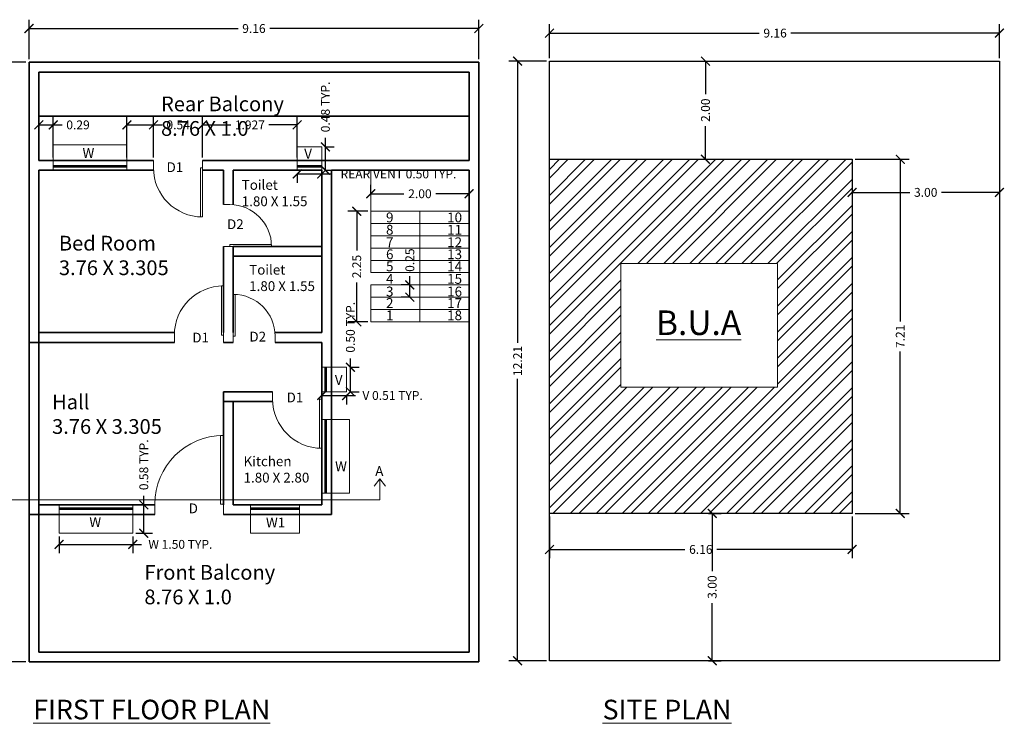
# Model space of a CAD drawing. Units: metres. Extents: x 6.8 to 74, y 0.6 to 37.
# Tile 3 of 5: x 20.1 to 40.1, y 4.1 to 18.4. Entities that reach past the tile are written whole.
import ezdxf

# ---------------------------------------------------------------- set-up
doc = ezdxf.new("R2010")
doc.units = ezdxf.units.M
doc.header["$LTSCALE"] = 0.2
doc.header["$MEASUREMENT"] = 0
for name, color, linetype, lineweight in [('A-ANNO-DIMS', 2, 'Continuous', 18), ('A-ANNO-SYMB', 3, 'Continuous', 18), ('A-ANNO-TEXT', 7, 'Continuous', 18), ('A-AREA-IDEN', 7, 'Continuous', 18), ('A-DOOR', 4, 'Continuous', 20), ('A-FLOR-STRS', 7, 'Continuous', 20), ('A-GLAZ', 4, 'Continuous', 18), ('A-SITE-BLDG', 7, 'Continuous', 25), ('A-WALL', 7, 'Continuous', 35), ('C-PROP', 3, 'Continuous', 30), ('C-SITE-PATT', 252, 'Continuous', 13)]:
    doc.layers.add(name, color=color, linetype=linetype, lineweight=lineweight)
doc.styles.get("Standard").update_dxf_attribs({"font": 'arial.ttf'})
doc.dimstyles.get("Standard").update_dxf_attribs({"dimtxt": 0.18, "dimasz": 0.18, "dimexe": 0.18, "dimexo": 0.0625, "dimgap": 0.09, "dimtad": 0, "dimzin": 0, "dimdsep": 46, "dimtxsty": 'Standard', "dimblk": 'ARCHTICK', "dimcen": 0.09, "dimadec": 0, "dimazin": 0, "dimtfac": 1, "dimtofl": 0, "dimtmove": 0, "dimatfit": 3, "dimfxl": 1, "dimfxlon": 1, "dimtolj": 1, "dimtzin": 0, "dimarcsym": 0})

# ---------------------------------------------------------------- blocks, each defined once
blk = doc.blocks.new('_ArchTick')
at = {"color": 0, "linetype": 'ByBlock', "const_width": 0.15}
blk.add_lwpolyline([(-0.5, -0.5), (0.5, 0.5)], dxfattribs=at)
blk = doc.blocks.new('*D5')
at = {"layer": 'A-ANNO-DIMS', "color": 0, "lineweight": -2, "transparency": 16777216}
for p, q in [((20.206, 17.556), (19.273, 17.556)), ((19.453, 17.556), (19.453, 11.819)), ((19.453, 5.346), (19.453, 11.083)), ((20.206, 5.346), (19.273, 5.346))]:
    blk.add_line(p, q, dxfattribs=at)
at = {"layer": 'Defpoints', "color": 0, "transparency": 16777216}
for p in [(20.268, 17.556), (19.453, 5.346), (20.268, 5.346)]:
    blk.add_point(p, dxfattribs=at)
at = {"layer": 'A-ANNO-DIMS', "color": 0, "lineweight": -2, "transparency": 16777216, "xscale": 0.18, "yscale": 0.18, "zscale": 0.18}
for p, rotation in [((19.453, 17.556), 90), ((19.453, 5.346), 270)]:
    blk.add_blockref('_ArchTick', p, dxfattribs=dict(at, rotation=rotation))
at = {"layer": 'A-ANNO-DIMS', "color": 0, "transparency": 16777216, "insert": (19.453, 11.451), "char_height": 0.18, "attachment_point": 5, "rotation": 90}
blk.add_mtext('\\A1;12.21', dxfattribs=at)
blk = doc.blocks.new('*D6')
at = {"layer": 'A-ANNO-DIMS', "color": 0, "lineweight": -2, "transparency": 16777216}
for p, q in [((20.268, 17.618), (20.268, 18.422)), ((29.428, 17.618), (29.428, 18.422)), ((20.268, 18.242), (24.525, 18.242)), ((29.428, 18.242), (25.172, 18.242))]:
    blk.add_line(p, q, dxfattribs=at)
at = {"layer": 'Defpoints', "color": 0, "transparency": 16777216}
for p in [(29.428, 18.242), (20.268, 17.556), (29.428, 17.556)]:
    blk.add_point(p, dxfattribs=at)
at = {"layer": 'A-ANNO-DIMS', "color": 0, "lineweight": -2, "transparency": 16777216, "xscale": 0.18, "yscale": 0.18, "zscale": 0.18, "rotation": 180}
blk.add_blockref('_ArchTick', (20.268, 18.242), dxfattribs=at)
at = {"layer": 'A-ANNO-DIMS', "color": 0, "lineweight": -2, "transparency": 16777216, "xscale": 0.18, "yscale": 0.18, "zscale": 0.18}
blk.add_blockref('_ArchTick', (29.428, 18.242), dxfattribs=at)
at = {"layer": 'A-ANNO-DIMS', "color": 0, "transparency": 16777216, "insert": (24.848, 18.242), "char_height": 0.18, "attachment_point": 5}
blk.add_mtext('\\A1;9.16', dxfattribs=at)
blk = doc.blocks.new('*U4')
for p, q in [((0, 0), (0, -6)), ((40, 0), (40, -6))]:
    blk.add_line(p, q)
blk.add_lwpolyline([(0, 0), (0, 40), (1.75, 40), (1.75, 0)], close=True)
blk.add_arc((0, 0), 40, 0, 90)
blk = doc.blocks.new('*D8')
at = {"layer": 'A-ANNO-DIMS', "color": 0, "lineweight": -2, "transparency": 16777216}
for p, q in [((37.091, 15.579), (38.189, 15.579)), ((38.009, 15.579), (38.009, 12.279)), ((38.009, 8.369), (38.009, 11.668)), ((37.091, 8.369), (38.189, 8.369))]:
    blk.add_line(p, q, dxfattribs=at)
at = {"layer": 'Defpoints', "color": 0, "transparency": 16777216}
for p in [(37.028, 15.579), (37.028, 8.369), (38.009, 8.369)]:
    blk.add_point(p, dxfattribs=at)
at = {"layer": 'A-ANNO-DIMS', "color": 0, "lineweight": -2, "transparency": 16777216, "xscale": 0.18, "yscale": 0.18, "zscale": 0.18}
for p, rotation in [((38.009, 15.579), 90), ((38.009, 8.369), 270)]:
    blk.add_blockref('_ArchTick', p, dxfattribs=dict(at, rotation=rotation))
at = {"layer": 'A-ANNO-DIMS', "color": 0, "transparency": 16777216, "insert": (38.009, 11.974), "char_height": 0.18, "attachment_point": 5, "rotation": 90}
blk.add_mtext('\\A1;7.21', dxfattribs=at)
blk = doc.blocks.new('*D9')
at = {"layer": 'A-ANNO-DIMS', "color": 0, "lineweight": -2, "transparency": 16777216}
for p, q in [((34.011, 17.579), (34.222, 17.579)), ((34.042, 17.579), (34.042, 16.904)), ((34.042, 15.579), (34.042, 16.254)), ((34.011, 15.579), (34.222, 15.579))]:
    blk.add_line(p, q, dxfattribs=at)
at = {"layer": 'Defpoints', "color": 0, "transparency": 16777216}
for p in [(33.948, 17.579), (34.042, 17.579), (33.948, 15.579)]:
    blk.add_point(p, dxfattribs=at)
at = {"layer": 'A-ANNO-DIMS', "color": 0, "lineweight": -2, "transparency": 16777216, "xscale": 0.18, "yscale": 0.18, "zscale": 0.18}
for p, rotation in [((34.042, 17.579), 90), ((34.042, 15.579), 270)]:
    blk.add_blockref('_ArchTick', p, dxfattribs=dict(at, rotation=rotation))
at = {"layer": 'A-ANNO-DIMS', "color": 0, "transparency": 16777216, "insert": (34.042, 16.579), "char_height": 0.18, "attachment_point": 5, "rotation": 90}
blk.add_mtext('\\A1;2.00', dxfattribs=at)
blk = doc.blocks.new('*D10')
at = {"layer": 'A-ANNO-DIMS', "color": 0, "lineweight": -2, "transparency": 16777216}
for p, q in [((34.104, 8.369), (34.359, 8.369)), ((34.179, 8.369), (34.179, 7.192)), ((34.179, 5.369), (34.179, 6.545)), ((34.104, 5.369), (34.359, 5.369))]:
    blk.add_line(p, q, dxfattribs=at)
at = {"layer": 'Defpoints', "color": 0, "transparency": 16777216}
for p in [(34.042, 8.369), (34.042, 5.369), (34.179, 5.369)]:
    blk.add_point(p, dxfattribs=at)
at = {"layer": 'A-ANNO-DIMS', "color": 0, "lineweight": -2, "transparency": 16777216, "xscale": 0.18, "yscale": 0.18, "zscale": 0.18}
for p, rotation in [((34.179, 8.369), 90), ((34.179, 5.369), 270)]:
    blk.add_blockref('_ArchTick', p, dxfattribs=dict(at, rotation=rotation))
at = {"layer": 'A-ANNO-DIMS', "color": 0, "transparency": 16777216, "insert": (34.179, 6.869), "char_height": 0.18, "attachment_point": 5, "rotation": 90}
blk.add_mtext('\\A1;3.00', dxfattribs=at)
blk = doc.blocks.new('*D11')
at = {"layer": 'A-ANNO-DIMS', "color": 0, "lineweight": -2, "transparency": 16777216}
for p, q in [((37.028, 15.001), (37.028, 14.726)), ((37.028, 14.906), (38.205, 14.906)), ((40.028, 14.906), (38.852, 14.906)), ((40.028, 15.001), (40.028, 14.726))]:
    blk.add_line(p, q, dxfattribs=at)
at = {"layer": 'Defpoints', "color": 0, "transparency": 16777216}
for p in [(37.028, 15.063), (40.028, 15.063), (40.028, 14.906)]:
    blk.add_point(p, dxfattribs=at)
at = {"layer": 'A-ANNO-DIMS', "color": 0, "lineweight": -2, "transparency": 16777216, "xscale": 0.18, "yscale": 0.18, "zscale": 0.18, "rotation": 180}
blk.add_blockref('_ArchTick', (37.028, 14.906), dxfattribs=at)
at = {"layer": 'A-ANNO-DIMS', "color": 0, "lineweight": -2, "transparency": 16777216, "xscale": 0.18, "yscale": 0.18, "zscale": 0.18}
blk.add_blockref('_ArchTick', (40.028, 14.906), dxfattribs=at)
at = {"layer": 'A-ANNO-DIMS', "color": 0, "transparency": 16777216, "insert": (38.528, 14.906), "char_height": 0.18, "attachment_point": 5}
blk.add_mtext('\\A1;3.00', dxfattribs=at)
blk = doc.blocks.new('*D12')
at = {"layer": 'A-ANNO-DIMS', "color": 0, "lineweight": -2, "transparency": 16777216}
for p, q in [((30.868, 17.641), (30.868, 18.329)), ((40.028, 17.641), (40.028, 18.329)), ((30.868, 18.149), (35.136, 18.149)), ((40.028, 18.149), (35.784, 18.149))]:
    blk.add_line(p, q, dxfattribs=at)
at = {"layer": 'Defpoints', "color": 0, "transparency": 16777216}
for p in [(40.028, 18.149), (30.868, 17.579), (40.028, 17.579)]:
    blk.add_point(p, dxfattribs=at)
at = {"layer": 'A-ANNO-DIMS', "color": 0, "lineweight": -2, "transparency": 16777216, "xscale": 0.18, "yscale": 0.18, "zscale": 0.18, "rotation": 180}
blk.add_blockref('_ArchTick', (30.868, 18.149), dxfattribs=at)
at = {"layer": 'A-ANNO-DIMS', "color": 0, "lineweight": -2, "transparency": 16777216, "xscale": 0.18, "yscale": 0.18, "zscale": 0.18}
blk.add_blockref('_ArchTick', (40.028, 18.149), dxfattribs=at)
at = {"layer": 'A-ANNO-DIMS', "color": 0, "transparency": 16777216, "insert": (35.46, 18.149), "char_height": 0.18, "attachment_point": 5}
blk.add_mtext('\\A1;9.16', dxfattribs=at)
blk = doc.blocks.new('*D13')
at = {"layer": 'A-ANNO-DIMS', "color": 0, "lineweight": -2, "transparency": 16777216}
for p, q in [((30.806, 17.579), (30.037, 17.579)), ((30.217, 17.579), (30.217, 11.842)), ((30.217, 5.369), (30.217, 11.106)), ((30.806, 5.369), (30.037, 5.369))]:
    blk.add_line(p, q, dxfattribs=at)
at = {"layer": 'Defpoints', "color": 0, "transparency": 16777216}
for p in [(30.868, 17.579), (30.217, 5.369), (30.868, 5.369)]:
    blk.add_point(p, dxfattribs=at)
at = {"layer": 'A-ANNO-DIMS', "color": 0, "lineweight": -2, "transparency": 16777216, "xscale": 0.18, "yscale": 0.18, "zscale": 0.18}
for p, rotation in [((30.217, 17.579), 90), ((30.217, 5.369), 270)]:
    blk.add_blockref('_ArchTick', p, dxfattribs=dict(at, rotation=rotation))
at = {"layer": 'A-ANNO-DIMS', "color": 0, "transparency": 16777216, "insert": (30.217, 11.474), "char_height": 0.18, "attachment_point": 5, "rotation": 90}
blk.add_mtext('\\A1;12.21', dxfattribs=at)
blk = doc.blocks.new('*D20')
at = {"layer": 'A-ANNO-DIMS', "color": 0, "lineweight": -2, "ltscale": 0.9, "transparency": 16777216}
for p, q in [((27.228, 14.878), (27.228, 15.058)), ((29.228, 14.878), (29.228, 15.058)), ((27.228, 14.878), (27.903, 14.878)), ((29.228, 14.878), (28.553, 14.878))]:
    blk.add_line(p, q, dxfattribs=at)
at = {"layer": 'Defpoints', "color": 0, "ltscale": 0.9, "transparency": 16777216}
for p in [(27.228, 14.878), (27.228, 14.823), (29.228, 14.823)]:
    blk.add_point(p, dxfattribs=at)
at = {"layer": 'A-ANNO-DIMS', "color": 0, "lineweight": -2, "ltscale": 0.9, "transparency": 16777216, "xscale": 0.18, "yscale": 0.18, "zscale": 0.18, "rotation": 180}
blk.add_blockref('_ArchTick', (27.228, 14.878), dxfattribs=at)
at = {"layer": 'A-ANNO-DIMS', "color": 0, "lineweight": -2, "ltscale": 0.9, "transparency": 16777216, "xscale": 0.18, "yscale": 0.18, "zscale": 0.18}
blk.add_blockref('_ArchTick', (29.228, 14.878), dxfattribs=at)
at = {"layer": 'A-ANNO-DIMS', "color": 0, "ltscale": 0.9, "transparency": 16777216, "insert": (28.228, 14.878), "char_height": 0.18, "attachment_point": 5}
blk.add_mtext('\\A1;2.00', dxfattribs=at)
blk = doc.blocks.new('*D21')
at = {"layer": 'A-ANNO-DIMS', "color": 0, "lineweight": -2, "ltscale": 0.9, "transparency": 16777216}
for p, q in [((27.166, 14.521), (26.761, 14.521)), ((26.941, 14.521), (26.941, 13.722)), ((26.941, 12.271), (26.941, 13.07)), ((27.166, 12.271), (26.761, 12.271))]:
    blk.add_line(p, q, dxfattribs=at)
at = {"layer": 'Defpoints', "color": 0, "ltscale": 0.9, "transparency": 16777216}
for p in [(27.228, 14.521), (26.941, 12.271), (27.228, 12.271)]:
    blk.add_point(p, dxfattribs=at)
at = {"layer": 'A-ANNO-DIMS', "color": 0, "lineweight": -2, "ltscale": 0.9, "transparency": 16777216, "xscale": 0.18, "yscale": 0.18, "zscale": 0.18}
for p, rotation in [((26.941, 14.521), 90), ((26.941, 12.271), 270)]:
    blk.add_blockref('_ArchTick', p, dxfattribs=dict(at, rotation=rotation))
at = {"layer": 'A-ANNO-DIMS', "color": 0, "ltscale": 0.9, "transparency": 16777216, "insert": (26.941, 13.396), "char_height": 0.18, "attachment_point": 5, "rotation": 90}
blk.add_mtext('\\A1;2.25', dxfattribs=at)
blk = doc.blocks.new('*D22')
at = {"layer": 'A-ANNO-DIMS', "color": 0, "lineweight": -2, "ltscale": 0.9, "transparency": 16777216}
for p, q in [((28.023, 13.021), (28.023, 13.201)), ((28.023, 13.021), (27.843, 13.021)), ((28.023, 12.771), (28.023, 13.021)), ((28.023, 12.771), (27.843, 12.771))]:
    blk.add_line(p, q, dxfattribs=at)
at = {"layer": 'Defpoints', "color": 0, "ltscale": 0.9, "transparency": 16777216}
for p in [(28.023, 13.021), (28.023, 13.021), (28.023, 12.771)]:
    blk.add_point(p, dxfattribs=at)
at = {"layer": 'A-ANNO-DIMS', "color": 0, "lineweight": -2, "ltscale": 0.9, "transparency": 16777216, "xscale": 0.18, "yscale": 0.18, "zscale": 0.18}
for p, rotation in [((28.023, 13.021), 90), ((28.023, 12.771), 270)]:
    blk.add_blockref('_ArchTick', p, dxfattribs=dict(at, rotation=rotation))
at = {"layer": 'A-ANNO-DIMS', "color": 0, "ltscale": 0.9, "transparency": 16777216, "insert": (28.023, 13.526), "char_height": 0.18, "attachment_point": 5, "rotation": 90}
blk.add_mtext('\\A1;0.25', dxfattribs=at)
blk = doc.blocks.new('WIN-W-1500-FRONT')
for p, q in [((0, 0.582), (0, 0.382)), ((0, 0.522), (1.5, 0.522)), ((0, 0.502), (1.5, 0.502)), ((0, 0.482), (1.5, 0.482)), ((1.5, 0.582), (1.5, 0.382)), ((0, 0), (0, 0.382)), ((1.5, 0.382), (1.5, 0)), ((1.5, 0), (0, 0))]:
    blk.add_line(p, q)
blk = doc.blocks.new('WIN-W1-1000-FRONT')
for p, q in [((0, 0.576), (0, 0.376)), ((1, 0.516), (0, 0.516)), ((1, 0.496), (0, 0.496)), ((1, 0.476), (0, 0.476)), ((1, 0.576), (1, 0.376)), ((0, 0), (0, 0.376)), ((1, 0.376), (1, 0)), ((1, 0), (0, 0))]:
    blk.add_line(p, q)
blk = doc.blocks.new('WIN-W-1500-SIDE')
for p, q in [((0, 1.5), (0.2, 1.5)), ((0.06, 0), (0.06, 1.5)), ((0.08, 0), (0.08, 1.5)), ((0.1, 0), (0.1, 1.5)), ((0.2, 1.5), (0.564, 1.5)), ((0.564, 1.5), (0.564, 0)), ((0, 0), (0.2, 0)), ((0.564, 0), (0.2, 0))]:
    blk.add_line(p, q)
blk = doc.blocks.new('WIN-W-1500-REAR')
for p, q in [((0, 0.2), (0, 0.517)), ((0, 0.517), (1.5, 0.517)), ((1.5, 0.517), (1.5, 0.2)), ((0, 0), (0, 0.2)), ((1.5, 0.1), (0, 0.1)), ((1.5, 0.08), (0, 0.08)), ((1.5, 0.06), (0, 0.06)), ((1.5, 0), (1.5, 0.2))]:
    blk.add_line(p, q)
blk = doc.blocks.new('VENT-500-REAR')
for p, q in [((0, 0.2), (0, 0.477)), ((0, 0.477), (0.5, 0.477)), ((0.5, 0.477), (0.5, 0.2)), ((0, 0), (0, 0.2)), ((0.5, 0.1), (0, 0.1)), ((0.5, 0.08), (0, 0.08)), ((0.5, 0.06), (0, 0.06)), ((0.5, 0), (0.5, 0.2))]:
    blk.add_line(p, q)
blk = doc.blocks.new('VENT-500-SIDE')
for p, q in [((0, 0.5), (0.2, 0.5)), ((0.06, 0.5), (0.06, 0)), ((0.08, 0.5), (0.08, 0)), ((0.1, 0.5), (0.1, 0)), ((0.2, 0.5), (0.507, 0.5)), ((0.507, 0.5), (0.507, 0)), ((0, 0), (0.2, 0)), ((0.507, 0), (0.2, 0))]:
    blk.add_line(p, q)
blk = doc.blocks.new('SECTION-HEAD-A')
for p, q in [((0, 0.429), (-0.116, 0.275)), ((0, 0), (0, 0.429)), ((0, 0.429), (0.116, 0.275))]:
    blk.add_line(p, q)
at = {"insert": (-0.093, 0.684), "char_height": 0.2, "attachment_point": 1}
blk.add_mtext_dynamic_manual_height_columns('A', width=0.50915, gutter_width=1, heights=[0], dxfattribs=at)
blk = doc.blocks.new('*D34')
at = {"layer": 'A-ANNO-DIMS', "color": 0, "lineweight": -2, "ltscale": 0.9, "transparency": 16777216}
for p, q in [((20.88, 7.901), (20.88, 7.559)), ((22.38, 7.901), (22.38, 7.559)), ((20.88, 7.739), (22.38, 7.739)), ((22.38, 7.739), (22.56, 7.739))]:
    blk.add_line(p, q, dxfattribs=at)
at = {"layer": 'Defpoints', "color": 0, "ltscale": 0.9, "transparency": 16777216}
for p in [(20.88, 7.964), (22.38, 7.964), (22.38, 7.739)]:
    blk.add_point(p, dxfattribs=at)
at = {"layer": 'A-ANNO-DIMS', "color": 0, "lineweight": -2, "ltscale": 0.9, "transparency": 16777216, "xscale": 0.18, "yscale": 0.18, "zscale": 0.18, "rotation": 180}
blk.add_blockref('_ArchTick', (20.88, 7.739), dxfattribs=at)
at = {"layer": 'A-ANNO-DIMS', "color": 0, "lineweight": -2, "ltscale": 0.9, "transparency": 16777216, "xscale": 0.18, "yscale": 0.18, "zscale": 0.18}
blk.add_blockref('_ArchTick', (22.38, 7.739), dxfattribs=at)
at = {"layer": 'A-ANNO-DIMS', "color": 0, "ltscale": 0.9, "transparency": 16777216, "insert": (23.35, 7.739), "char_height": 0.18, "attachment_point": 5}
blk.add_mtext('\\A1;W 1.50 TYP.', dxfattribs=at)
blk = doc.blocks.new('*D35')
at = {"layer": 'A-ANNO-DIMS', "color": 0, "lineweight": -2, "ltscale": 0.9, "transparency": 16777216}
for p, q in [((22.605, 8.546), (22.605, 8.726)), ((22.443, 8.546), (22.785, 8.546)), ((22.605, 7.964), (22.605, 8.546)), ((22.443, 7.964), (22.785, 7.964))]:
    blk.add_line(p, q, dxfattribs=at)
at = {"layer": 'Defpoints', "color": 0, "ltscale": 0.9, "transparency": 16777216}
for p in [(22.38, 8.546), (22.605, 8.546), (22.38, 7.964)]:
    blk.add_point(p, dxfattribs=at)
at = {"layer": 'A-ANNO-DIMS', "color": 0, "lineweight": -2, "ltscale": 0.9, "transparency": 16777216, "xscale": 0.18, "yscale": 0.18, "zscale": 0.18}
for p, rotation in [((22.605, 8.546), 90), ((22.605, 7.964), 270)]:
    blk.add_blockref('_ArchTick', p, dxfattribs=dict(at, rotation=rotation))
at = {"layer": 'A-ANNO-DIMS', "color": 0, "ltscale": 0.9, "transparency": 16777216, "insert": (22.605, 9.359), "char_height": 0.18, "attachment_point": 5, "rotation": 90}
blk.add_mtext('\\A1;0.58 TYP.', dxfattribs=at)
blk = doc.blocks.new('*D42')
at = {"layer": 'A-ANNO-DIMS', "color": 0, "lineweight": -2, "ltscale": 0.9, "transparency": 16777216}
for p, q in [((25.728, 15.293), (25.728, 15.101)), ((25.728, 15.281), (26.228, 15.281)), ((26.228, 15.293), (26.228, 15.101)), ((26.228, 15.281), (26.408, 15.281))]:
    blk.add_line(p, q, dxfattribs=at)
at = {"layer": 'Defpoints', "color": 0, "ltscale": 0.9, "transparency": 16777216}
for p in [(25.728, 15.356), (26.228, 15.356), (26.228, 15.281)]:
    blk.add_point(p, dxfattribs=at)
at = {"layer": 'A-ANNO-DIMS', "color": 0, "lineweight": -2, "ltscale": 0.9, "transparency": 16777216, "xscale": 0.18, "yscale": 0.18, "zscale": 0.18, "rotation": 180}
blk.add_blockref('_ArchTick', (25.728, 15.281), dxfattribs=at)
at = {"layer": 'A-ANNO-DIMS', "color": 0, "lineweight": -2, "ltscale": 0.9, "transparency": 16777216, "xscale": 0.18, "yscale": 0.18, "zscale": 0.18}
blk.add_blockref('_ArchTick', (26.228, 15.281), dxfattribs=at)
at = {"layer": 'A-ANNO-DIMS', "color": 0, "ltscale": 0.9, "transparency": 16777216, "insert": (27.791, 15.281), "char_height": 0.18, "attachment_point": 5}
blk.add_mtext('\\A1;REAR VENT 0.50 TYP.', dxfattribs=at)
blk = doc.blocks.new('*D43')
at = {"layer": 'A-ANNO-DIMS', "color": 0, "lineweight": -2, "ltscale": 0.9, "transparency": 16777216}
for p, q in [((26.303, 15.833), (26.303, 16.013)), ((26.291, 15.833), (26.483, 15.833)), ((26.303, 15.356), (26.303, 15.833)), ((26.291, 15.356), (26.483, 15.356))]:
    blk.add_line(p, q, dxfattribs=at)
at = {"layer": 'Defpoints', "color": 0, "ltscale": 0.9, "transparency": 16777216}
for p in [(26.228, 15.833), (26.303, 15.833), (26.228, 15.356)]:
    blk.add_point(p, dxfattribs=at)
at = {"layer": 'A-ANNO-DIMS', "color": 0, "lineweight": -2, "ltscale": 0.9, "transparency": 16777216, "xscale": 0.18, "yscale": 0.18, "zscale": 0.18}
for p, rotation in [((26.303, 15.833), 90), ((26.303, 15.356), 270)]:
    blk.add_blockref('_ArchTick', p, dxfattribs=dict(at, rotation=rotation))
at = {"layer": 'A-ANNO-DIMS', "color": 0, "ltscale": 0.9, "transparency": 16777216, "insert": (26.303, 16.646), "char_height": 0.18, "attachment_point": 5, "rotation": 90}
blk.add_mtext('\\A1;0.48 TYP.', dxfattribs=at)
blk = doc.blocks.new('*D44')
at = {"layer": 'A-ANNO-DIMS', "color": 0, "lineweight": -2, "ltscale": 0.9, "transparency": 16777216}
for p, q in [((26.228, 10.783), (26.228, 10.59)), ((26.228, 10.77), (26.736, 10.77)), ((26.736, 10.783), (26.736, 10.59)), ((26.736, 10.77), (26.916, 10.77))]:
    blk.add_line(p, q, dxfattribs=at)
at = {"layer": 'Defpoints', "color": 0, "ltscale": 0.9, "transparency": 16777216}
for p in [(26.228, 10.846), (26.736, 10.846), (26.736, 10.77)]:
    blk.add_point(p, dxfattribs=at)
at = {"layer": 'A-ANNO-DIMS', "color": 0, "lineweight": -2, "ltscale": 0.9, "transparency": 16777216, "xscale": 0.18, "yscale": 0.18, "zscale": 0.18, "rotation": 180}
blk.add_blockref('_ArchTick', (26.228, 10.77), dxfattribs=at)
at = {"layer": 'A-ANNO-DIMS', "color": 0, "lineweight": -2, "ltscale": 0.9, "transparency": 16777216, "xscale": 0.18, "yscale": 0.18, "zscale": 0.18}
blk.add_blockref('_ArchTick', (26.736, 10.77), dxfattribs=at)
at = {"layer": 'A-ANNO-DIMS', "color": 0, "ltscale": 0.9, "transparency": 16777216, "insert": (27.672, 10.77), "char_height": 0.18, "attachment_point": 5}
blk.add_mtext('\\A1;V 0.51 TYP.', dxfattribs=at)
blk = doc.blocks.new('*D45')
at = {"layer": 'A-ANNO-DIMS', "color": 0, "lineweight": -2, "ltscale": 0.9, "transparency": 16777216}
for p, q in [((26.812, 11.346), (26.812, 11.526)), ((26.798, 11.346), (26.992, 11.346)), ((26.812, 10.846), (26.812, 11.346)), ((26.798, 10.846), (26.992, 10.846))]:
    blk.add_line(p, q, dxfattribs=at)
at = {"layer": 'Defpoints', "color": 0, "ltscale": 0.9, "transparency": 16777216}
for p in [(26.736, 11.346), (26.812, 11.346), (26.736, 10.846)]:
    blk.add_point(p, dxfattribs=at)
at = {"layer": 'A-ANNO-DIMS', "color": 0, "lineweight": -2, "ltscale": 0.9, "transparency": 16777216, "xscale": 0.18, "yscale": 0.18, "zscale": 0.18}
for p, rotation in [((26.812, 11.346), 90), ((26.812, 10.846), 270)]:
    blk.add_blockref('_ArchTick', p, dxfattribs=dict(at, rotation=rotation))
at = {"layer": 'A-ANNO-DIMS', "color": 0, "ltscale": 0.9, "transparency": 16777216, "insert": (26.812, 12.159), "char_height": 0.18, "attachment_point": 5, "rotation": 90}
blk.add_mtext('\\A1;0.50 TYP.', dxfattribs=at)
blk = doc.blocks.new('*D59')
at = {"layer": 'A-ANNO-DIMS', "color": 0, "lineweight": -2, "ltscale": 0.9, "transparency": 16777216}
for p, q in [((30.868, 8.306), (30.868, 7.456)), ((37.028, 8.306), (37.028, 7.456)), ((30.868, 7.636), (33.624, 7.636)), ((37.028, 7.636), (34.273, 7.636))]:
    blk.add_line(p, q, dxfattribs=at)
at = {"layer": 'Defpoints', "color": 0, "ltscale": 0.9, "transparency": 16777216}
for p in [(30.868, 8.369), (37.028, 8.369), (30.868, 7.636)]:
    blk.add_point(p, dxfattribs=at)
at = {"layer": 'A-ANNO-DIMS', "color": 0, "lineweight": -2, "ltscale": 0.9, "transparency": 16777216, "xscale": 0.18, "yscale": 0.18, "zscale": 0.18, "rotation": 180}
blk.add_blockref('_ArchTick', (30.868, 7.636), dxfattribs=at)
at = {"layer": 'A-ANNO-DIMS', "color": 0, "lineweight": -2, "ltscale": 0.9, "transparency": 16777216, "xscale": 0.18, "yscale": 0.18, "zscale": 0.18}
blk.add_blockref('_ArchTick', (37.028, 7.636), dxfattribs=at)
at = {"layer": 'A-ANNO-DIMS', "color": 0, "ltscale": 0.9, "transparency": 16777216, "insert": (33.948, 7.636), "char_height": 0.18, "attachment_point": 5}
blk.add_mtext('\\A1;6.16', dxfattribs=at)
blk = doc.blocks.new('*D70')
at = {"layer": 'A-ANNO-DIMS', "color": 0, "lineweight": -2, "ltscale": 0.9, "transparency": 16777216}
for p, q in [((20.468, 15.618), (20.468, 16.46)), ((20.762, 15.618), (20.762, 16.46)), ((20.468, 16.28), (20.762, 16.28)), ((20.762, 16.28), (20.942, 16.28))]:
    blk.add_line(p, q, dxfattribs=at)
at = {"layer": 'Defpoints', "color": 0, "ltscale": 0.9, "transparency": 16777216}
for p in [(20.762, 16.28), (20.468, 15.556), (20.762, 15.556)]:
    blk.add_point(p, dxfattribs=at)
at = {"layer": 'A-ANNO-DIMS', "color": 0, "lineweight": -2, "ltscale": 0.9, "transparency": 16777216, "xscale": 0.18, "yscale": 0.18, "zscale": 0.18, "rotation": 180}
blk.add_blockref('_ArchTick', (20.468, 16.28), dxfattribs=at)
at = {"layer": 'A-ANNO-DIMS', "color": 0, "lineweight": -2, "ltscale": 0.9, "transparency": 16777216, "xscale": 0.18, "yscale": 0.18, "zscale": 0.18}
blk.add_blockref('_ArchTick', (20.762, 16.28), dxfattribs=at)
at = {"layer": 'A-ANNO-DIMS', "color": 0, "ltscale": 0.9, "transparency": 16777216, "insert": (21.266, 16.28), "char_height": 0.18, "attachment_point": 5}
blk.add_mtext('\\A1;0.29', dxfattribs=at)
blk = doc.blocks.new('*D71')
at = {"layer": 'A-ANNO-DIMS', "color": 0, "lineweight": -2, "ltscale": 0.9, "transparency": 16777216}
for p, q in [((22.262, 15.618), (22.262, 16.46)), ((22.802, 15.618), (22.802, 16.46)), ((22.262, 16.28), (22.802, 16.28)), ((22.802, 16.28), (22.982, 16.28))]:
    blk.add_line(p, q, dxfattribs=at)
at = {"layer": 'Defpoints', "color": 0, "ltscale": 0.9, "transparency": 16777216}
for p in [(22.802, 16.28), (22.262, 15.556), (22.802, 15.556)]:
    blk.add_point(p, dxfattribs=at)
at = {"layer": 'A-ANNO-DIMS', "color": 0, "lineweight": -2, "ltscale": 0.9, "transparency": 16777216, "xscale": 0.18, "yscale": 0.18, "zscale": 0.18, "rotation": 180}
blk.add_blockref('_ArchTick', (22.262, 16.28), dxfattribs=at)
at = {"layer": 'A-ANNO-DIMS', "color": 0, "lineweight": -2, "ltscale": 0.9, "transparency": 16777216, "xscale": 0.18, "yscale": 0.18, "zscale": 0.18}
blk.add_blockref('_ArchTick', (22.802, 16.28), dxfattribs=at)
at = {"layer": 'A-ANNO-DIMS', "color": 0, "ltscale": 0.9, "transparency": 16777216, "insert": (23.305, 16.28), "char_height": 0.18, "attachment_point": 5}
blk.add_mtext('\\A1;0.54', dxfattribs=at)
blk = doc.blocks.new('*D72')
at = {"layer": 'A-ANNO-DIMS', "color": 0, "lineweight": -2, "ltscale": 0.9, "transparency": 16777216}
for p, q in [((23.802, 15.618), (23.802, 16.46)), ((25.728, 15.618), (25.728, 16.46)), ((23.802, 16.28), (24.38, 16.28)), ((25.728, 16.28), (25.15, 16.28))]:
    blk.add_line(p, q, dxfattribs=at)
at = {"layer": 'Defpoints', "color": 0, "ltscale": 0.9, "transparency": 16777216}
for p in [(25.728, 16.28), (23.802, 15.556), (25.728, 15.556)]:
    blk.add_point(p, dxfattribs=at)
at = {"layer": 'A-ANNO-DIMS', "color": 0, "lineweight": -2, "ltscale": 0.9, "transparency": 16777216, "xscale": 0.18, "yscale": 0.18, "zscale": 0.18, "rotation": 180}
blk.add_blockref('_ArchTick', (23.802, 16.28), dxfattribs=at)
at = {"layer": 'A-ANNO-DIMS', "color": 0, "lineweight": -2, "ltscale": 0.9, "transparency": 16777216, "xscale": 0.18, "yscale": 0.18, "zscale": 0.18}
blk.add_blockref('_ArchTick', (25.728, 16.28), dxfattribs=at)
at = {"layer": 'A-ANNO-DIMS', "color": 0, "ltscale": 0.9, "transparency": 16777216, "insert": (24.765, 16.28), "char_height": 0.18, "attachment_point": 5}
blk.add_mtext('\\A1;1.927', dxfattribs=at)

msp = doc.modelspace()

# ---------------------------------------------------------------- hatches: boundary and pattern name
at = {"layer": 'C-SITE-PATT'}
h = msp.add_hatch(dxfattribs=at)
h.set_pattern_fill('ANSI32', color=256)
h.set_pattern_definition([(45, (0, -0.6447), (-0.265165, 0.265165), []), (45, (0.17678, -0.6447), (-0.265165, 0.265165), [])])
h.paths.add_polyline_path([(37.0283, 8.3687), (37.0283, 15.5787), (30.8683, 15.5787), (30.8683, 8.3687)])
h.paths.add_polyline_path([(32.3223, 10.9383), (32.3223, 13.4561), (35.5104, 13.4561), (35.5104, 10.9383)], flags=16)
h.paths.add_polyline_path([(32.8592, 11.7289), (34.9345, 11.7289), (34.9345, 12.7592), (32.8592, 12.7592)], flags=8)

# ---------------------------------------------------------------- linework, layer by layer
at = {"layer": 'A-ANNO-SYMB'}
msp.add_line((27.4115, 8.6471), (19.8042, 8.6471), dxfattribs=at)
at = {"layer": 'A-AREA-IDEN'}
msp.add_lwpolyline([(32.3223, 13.4561), (35.5104, 13.4561), (35.5104, 10.9383), (32.3223, 10.9383)], close=True, dxfattribs=at)
at = {"layer": 'A-FLOR-STRS'}
for p, q in [((27.2285, 13.2715), (27.2285, 15.3558)), ((29.2285, 14.5215), (27.2285, 14.5215)), ((28.2285, 12.2715), (28.2285, 14.5215)), ((29.2285, 14.2715), (27.2285, 14.2715)), ((29.2285, 14.0215), (27.2285, 14.0215)), ((29.2285, 13.7715), (27.2285, 13.7715)), ((29.2285, 13.5215), (27.2285, 13.5215)), ((29.2285, 13.2715), (27.2285, 13.2715)), ((29.2285, 13.0215), (27.2285, 13.0215)), ((27.2285, 12.2715), (27.2285, 13.0215)), ((29.2285, 12.7715), (27.2285, 12.7715)), ((29.2285, 12.5215), (27.2285, 12.5215)), ((29.2285, 12.2715), (27.2285, 12.2715))]:
    msp.add_line(p, q, dxfattribs=at)
at = {"layer": 'A-SITE-BLDG'}
for p, q in [((30.8683, 15.5787), (37.0283, 15.5787)), ((37.0283, 15.5787), (37.0283, 8.3687)), ((37.0283, 8.3687), (30.8683, 8.3687))]:
    msp.add_line(p, q, dxfattribs=at)
at = {"layer": 'A-WALL'}
for p, q in [((20.2685, 17.5558), (29.4285, 17.5558)), ((20.2685, 17.5558), (20.2685, 5.3458)), ((29.4285, 17.5558), (29.4285, 5.3458)), ((20.4685, 17.3558), (29.2285, 17.3558)), ((20.4685, 17.3558), (20.4685, 15.5558)), ((29.2285, 17.3558), (29.2285, 15.5558)), ((20.4685, 16.4558), (29.2285, 16.4558)), ((20.4685, 15.5558), (22.8016, 15.5558)), ((23.8016, 15.5558), (29.2285, 15.5558)), ((20.4685, 15.3558), (22.8028, 15.3558)), ((20.4685, 15.3558), (20.4685, 5.5458)), ((23.8016, 15.3558), (24.2285, 15.3558)), ((24.2285, 15.3558), (24.2285, 14.6558)), ((24.4285, 15.3558), (26.2285, 15.3558)), ((24.4285, 15.3558), (24.4285, 14.6527)), ((26.2285, 15.3558), (26.2285, 12.0508)), ((26.4285, 15.3558), (29.2285, 15.3558)), ((26.4285, 15.3558), (26.4285, 8.3458)), ((29.2285, 15.3558), (29.2285, 5.5458)), ((24.2285, 13.8058), (24.2285, 12.0508)), ((24.4285, 13.8058), (26.2285, 13.8058)), ((24.4285, 13.8058), (24.4285, 12.0508)), ((24.4285, 13.6058), (26.2285, 13.6058)), ((20.4685, 12.0508), (23.2297, 12.0508)), ((25.2754, 12.0508), (26.2285, 12.0508)), ((20.2685, 11.8508), (23.2285, 11.8508)), ((24.2285, 11.8508), (24.4285, 11.8508)), ((25.2785, 11.8508), (26.2285, 11.8508)), ((26.2285, 11.8508), (26.2285, 8.5458)), ((24.2285, 10.8458), (25.2285, 10.8458)), ((24.2285, 10.8458), (24.2285, 8.5458)), ((24.2285, 10.6458), (25.2297, 10.6458)), ((24.4285, 10.6458), (24.4285, 8.5458)), ((20.4685, 8.5458), (22.8285, 8.5458)), ((24.4285, 8.5458), (26.2285, 8.5458)), ((20.2685, 8.3458), (22.8285, 8.3458)), ((24.2285, 8.3458), (26.4285, 8.3458)), ((20.4685, 5.5458), (29.2285, 5.5458)), ((20.2685, 5.3458), (29.4285, 5.3458))]:
    msp.add_line(p, q, dxfattribs=at)
at = {"layer": 'C-PROP'}
for p, q in [((30.8683, 17.5787), (40.0283, 17.5787)), ((30.8683, 5.3687), (30.8683, 17.5787)), ((40.0283, 17.5787), (40.0283, 5.3687)), ((40.0283, 5.3687), (30.8683, 5.3687))]:
    msp.add_line(p, q, dxfattribs=at)

# ---------------------------------------------------------------- block references
at = {"layer": 'A-ANNO-SYMB'}
msp.add_blockref('SECTION-HEAD-A', (27.4115, 8.6471), dxfattribs=at)
at = {"layer": 'A-DOOR'}
for p, xscale, yscale, zscale, rotation in [((23.8016, 15.4058), 0.025, 0.025, 0.025, 180), ((24.356, 13.8058), -0.02125, 0.02125, 0.02125, 270), ((26.2285, 10.6958), 0.025, 0.025, 0.025, 180)]:
    msp.add_blockref('*U4', p, dxfattribs=dict(at, xscale=xscale, yscale=yscale, zscale=zscale, rotation=rotation))
for p, xscale, yscale, zscale in [((24.2285, 12.0008), -0.025, 0.025, 0.025), ((24.4285, 11.9783), 0.02125, 0.02125, 0.02125), ((24.2285, 8.5558), -0.0350000000000001, 0.0350000000000001, 0.0350000000000001)]:
    msp.add_blockref('*U4', p, dxfattribs=dict(at, xscale=xscale, yscale=yscale, zscale=zscale))
at = {"layer": 'A-GLAZ'}
for name, p in [('WIN-W-1500-REAR', (20.7619, 15.3558)), ('VENT-500-REAR', (25.7285, 15.3558)), ('VENT-500-SIDE', (26.2285, 10.8458)), ('WIN-W-1500-SIDE', (26.2285, 8.7794)), ('WIN-W-1500-FRONT', (20.8803, 7.9638)), ('WIN-W1-1000-FRONT', (24.7757, 7.97))]:
    msp.add_blockref(name, p, dxfattribs=at)

# ---------------------------------------------------------------- texts
at = {"layer": 'A-ANNO-TEXT', "attachment_point": 1}
for s, width, heights, insert, char_height in [('W', 0.509148, [0], (21.3578, 15.8073), 0.2), ('V', 0.509148, [0], (25.8721, 15.7928), 0.2), ('D1', 0.509148, [0], (23.069, 15.5181), 0.2), ('9', 1.417327, [0], (27.5381, 14.4953), 0.2), ('10', 1.417327, [0], (28.7831, 14.4953), 0.2), ('D2', 0.509148, [0], (24.3001, 14.3576), 0.2), ('8', 1.417327, [0], (27.5381, 14.2442), 0.2), ('11', 1.417327, [0], (28.7831, 14.2442), 0.2), ('7', 1.417327, [0], (27.5381, 13.9899), 0.2), ('12', 1.417327, [0], (28.7831, 13.9899), 0.2), ('6', 1.417327, [0], (27.5381, 13.7457), 0.2), ('13', 1.417327, [0], (28.7831, 13.7457), 0.2), ('5', 1.417327, [0], (27.5381, 13.4997), 0.2), ('14', 1.417327, [0], (28.7831, 13.4997), 0.2), ('4', 1.417327, [0], (27.5381, 13.2441), 0.2), ('15', 1.417327, [0], (28.7831, 13.2441), 0.2), ('3', 1.417327, [0], (27.5381, 12.9872), 0.2), ('16', 1.417327, [0], (28.7831, 12.9872), 0.2), ('2', 1.417327, [0], (27.5381, 12.7522), 0.2), ('17', 1.417327, [0], (28.7831, 12.7522), 0.2), ('1', 1.417327, [0], (27.5381, 12.5019), 0.2), ('18', 1.417327, [0], (28.7831, 12.5019), 0.2), ('D1', 0.509148, [0], (23.5935, 12.0492), 0.2), ('D2', 0.509148, [0], (24.756, 12.0693), 0.2), ('V', 0.509148, [0], (26.4954, 11.1869), 0.2), ('D1', 0.509148, [0], (25.5134, 10.83), 0.2), ('W', 0.509148, [0], (26.5015, 9.4281), 0.2), ('D', 0.509148, [0], (23.5197, 8.5717), 0.2), ('W', 0.509148, [0], (21.4967, 8.2919), 0.2), ('W1', 0.509148, [0], (25.0932, 8.2826), 0.2), ('{\\LFIRST FLOOR PLAN}', 7.004508, [0], (20.3539, 4.5755), 0.4), ('{\\LSITE PLAN}', 7.004508, [0.4871], (31.948, 4.5755), 0.4)]:
    msp.add_mtext_dynamic_manual_height_columns(s, width=width, gutter_width=1, heights=heights, dxfattribs=dict(at, insert=insert, char_height=char_height))
at = {"layer": 'A-AREA-IDEN', "attachment_point": 1}
for s, width, heights, insert, char_height in [('Rear Balcony\\P8.76 X 1.0', 6.143632, [0], (22.9561, 16.8575), 0.3), ('Toilet\\P1.80 X 1.55', 1.743148, [0], (24.5996, 15.1577), 0.2), ('Bed Room\\P3.76 X 3.305', 3.423868, [0], (20.8765, 14.0211), 0.3), ('Toilet\\P1.80 X 1.55', 1.743148, [0], (24.7515, 13.4302), 0.2), ('{\\LB.U.A}', 2.00964, [0.4871], (33.0353, 12.5019), 0.5), ('Hall\\P3.76 X 3.305', 6.143632, [0], (20.738, 10.789), 0.3), ('Kitchen\\P1.80 X 2.80', 1.743148, [0], (24.637, 9.531), 0.2), ('Front Balcony\\P8.76 X 1.0', 3.328114, [0], (22.6175, 7.3187), 0.3)]:
    msp.add_mtext_dynamic_manual_height_columns(s, width=width, gutter_width=1, heights=heights, dxfattribs=dict(at, insert=insert, char_height=char_height))

# ---------------------------------------------------------------- dimensions: what is measured, and where the dimension line sits
at = {"layer": 'A-ANNO-DIMS'}
for base, p1, p2, picture, middle in [((29.4285, 18.2416), (20.2685, 17.5558), (29.4285, 17.5558), '*D6', (24.8485, 18.2416)), ((40.0283, 14.9065), (37.0283, 15.0635), (40.0283, 15.0635), '*D11', (38.5283, 14.9065))]:
    dim = msp.add_linear_dim(base=base, p1=p1, p2=p2, dimstyle='Standard', override={"dimclrd": 0, "dimclre": 0, "dimclrt": 0}, dxfattribs=at)
    dim.commit()
    dim.dimension.update_dxf_attribs({"geometry": picture, "text_midpoint": middle})
dim = msp.add_linear_dim(base=(40.0283, 18.1491), p1=(30.8683, 17.5787), p2=(40.0283, 17.5787), dimstyle='Standard', override={"dimclrd": 0, "dimclre": 0, "dimclrt": 0}, dxfattribs=at)
dim.commit()
dim.dimension.update_dxf_attribs({"geometry": '*D12', "text_midpoint": (35.4601, 18.1491), "dimtype": 160})
for base, p1, p2, picture, middle in [((19.4535, 5.3458), (20.2685, 17.5558), (20.2685, 5.3458), '*D5', (19.4535, 11.4508)), ((30.2173, 5.3687), (30.8683, 17.5787), (30.8683, 5.3687), '*D13', (30.2173, 11.4737)), ((34.0416, 17.5787), (33.9483, 15.5787), (33.9483, 17.5787), '*D9', (34.0416, 16.5787)), ((38.0094, 8.3687), (37.0283, 15.5787), (37.0283, 8.3687), '*D8', (38.0094, 11.9737)), ((34.1788, 5.3687), (34.0416, 8.3687), (34.0416, 5.3687), '*D10', (34.1788, 6.8687))]:
    dim = msp.add_linear_dim(base=base, p1=p1, p2=p2, angle=90, dimstyle='Standard', override={"dimclrd": 0, "dimclre": 0, "dimclrt": 0}, dxfattribs=at)
    dim.commit()
    dim.dimension.update_dxf_attribs({"geometry": picture, "text_midpoint": middle})
at = {"layer": 'A-ANNO-DIMS', "ltscale": 0.9}
for base, p1, p2, picture, middle in [((26.3035, 15.8328), (26.2285, 15.3558), (26.2285, 15.8328), '*D43', (26.3035, 16.6457)), ((26.8118, 11.3458), (26.7357, 10.8458), (26.7357, 11.3458), '*D45', (26.8118, 12.1587)), ((22.6053, 8.5458), (22.3803, 7.9638), (22.3803, 8.5458), '*D35', (22.6053, 9.3587))]:
    dim = msp.add_linear_dim(base=base, p1=p1, p2=p2, angle=90, text='<> TYP.', dimstyle='Standard', override={"dimdec": 2, "dimlfac": 1, "dimrnd": 0, "dimzin": 0, "dimdsep": 46, "dimlunit": 2}, dxfattribs=at)
    dim.commit()
    dim.dimension.update_dxf_attribs({"geometry": picture, "text_midpoint": middle})
for base, p1, p2, angle, override, picture, middle in [((20.7619, 16.2803), (20.4685, 15.5558), (20.7619, 15.5558), 0, {"dimdec": 2, "dimlfac": 1, "dimrnd": 0, "dimzin": 0, "dimdsep": 46, "dimlunit": 2}, '*D70', (21.2659, 16.2803)), ((25.7285, 16.2803), (23.8016, 15.5558), (25.7285, 15.5558), 0, {"dimdec": 3, "dimlfac": 1, "dimrnd": 0, "dimzin": 0, "dimdsep": 46, "dimlunit": 2}, '*D72', (24.765, 16.2803)), ((26.941, 12.2715), (27.2285, 14.5215), (27.2285, 12.2715), 90, {"dimclrd": 0, "dimclre": 0, "dimclrt": 0}, '*D21', (26.941, 13.3965)), ((28.0228, 13.0215), (28.0228, 12.7715), (28.0228, 13.0215), 90, {"dimclrd": 0, "dimclre": 0, "dimclrt": 0}, '*D22', (28.0228, 13.5259)), ((30.8683, 7.6362), (37.0283, 8.3687), (30.8683, 8.3687), 180, {"dimdec": 2, "dimlfac": 1, "dimrnd": 0, "dimzin": 0, "dimdsep": 46, "dimlunit": 2}, '*D59', (33.9483, 7.6362))]:
    dim = msp.add_linear_dim(base=base, p1=p1, p2=p2, angle=angle, dimstyle='Standard', override=override, dxfattribs=at)
    dim.commit()
    dim.dimension.update_dxf_attribs({"geometry": picture, "text_midpoint": middle})
for base, p1, p2, override, picture, middle in [((22.8016, 16.2803), (22.2619, 15.5558), (22.8016, 15.5558), {"dimdec": 2, "dimlfac": 1, "dimrnd": 0, "dimzin": 0, "dimdsep": 46, "dimlunit": 2}, '*D71', (23.305, 16.2803)), ((27.2285, 14.8783), (29.2285, 14.8229), (27.2285, 14.8229), {"dimclrd": 0, "dimclre": 0, "dimclrt": 0}, '*D20', (28.2285, 14.8783))]:
    dim = msp.add_linear_dim(base=base, p1=p1, p2=p2, dimstyle='Standard', override=override, dxfattribs=at)
    dim.commit()
    dim.dimension.update_dxf_attribs({"geometry": picture, "text_midpoint": middle})
for base, p1, p2, text, picture, middle in [((26.2285, 15.2808), (25.7285, 15.3558), (26.2285, 15.3558), 'REAR VENT <> TYP.', '*D42', (27.7913, 15.2808)), ((26.7357, 10.7697), (26.2285, 10.8458), (26.7357, 10.8458), 'V <> TYP.', '*D44', (27.6721, 10.7697)), ((22.3803, 7.7388), (20.8803, 7.9638), (22.3803, 7.9638), 'W <> TYP.', '*D34', (23.3505, 7.7388))]:
    dim = msp.add_linear_dim(base=base, p1=p1, p2=p2, text=text, dimstyle='Standard', override={"dimdec": 2, "dimlfac": 1, "dimrnd": 0, "dimzin": 0, "dimdsep": 46, "dimlunit": 2}, dxfattribs=at)
    dim.commit()
    dim.dimension.update_dxf_attribs({"geometry": picture, "text_midpoint": middle})

doc.saveas('drawing.dxf')
